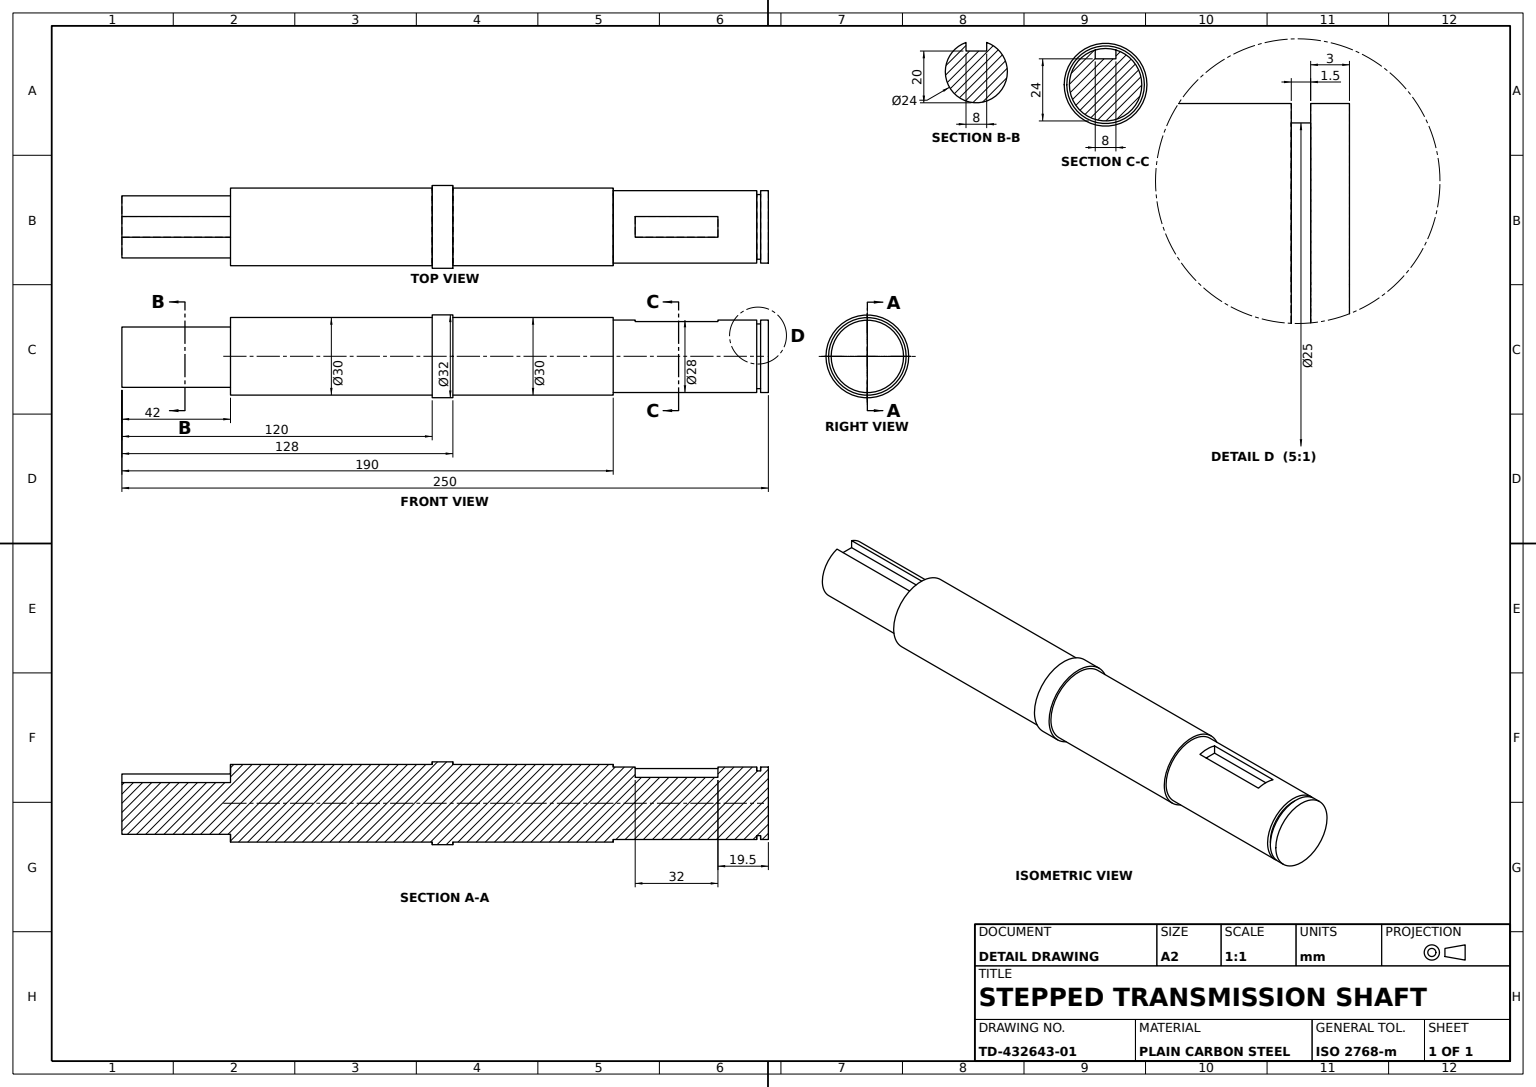
from build123d import *

# Parameters (mm, degrees)
KEYWAY_1_SKETCH_W  = 42
KEYWAY_1_SKETCH_H  = 8
KEYWAY_1_CUT_DEPTH = 4
KEYWAY_2_SKETCH_W  = 32
KEYWAY_2_SKETCH_H  = 8
KEYWAY_2_CUT_DEPTH = 4


with BuildPart() as part:
    # Shaft Profile Sketch → Stepped Shaft Body (revolve)
    with BuildSketch(Plane.XY, mode=Mode.PRIVATE) as stepped_shaft_body_sk:
        Polygon((0, 0), (0, 12), (42, 12), (42, 15), (120, 15), (120, 16), (128, 16), (128, 15), (190, 15), (190, 14), (245.5, 14), (245.5, 12.5), (247, 12.5), (247, 14), (250, 14), (250, 0), align=None)
    revolve(stepped_shaft_body_sk.sketch.rotate(Axis((0, 0, 0), (1, 0, 0)), 90), axis=Axis((0, 0, 0), (1, 0, 0)))

    # Keyway 1 Sketch → Keyway 1 Cut (cut)
    with BuildSketch(Plane(origin=(0, 12, 0), x_dir=(1, 0, 0), z_dir=(0, 1, 0))):
        with Locations((21, 0)):
            Rectangle(KEYWAY_1_SKETCH_W, KEYWAY_1_SKETCH_H)
    extrude(amount=-KEYWAY_1_CUT_DEPTH, mode=Mode.SUBTRACT)

    # Keyway 2 Sketch → Keyway 2 Cut (cut)
    with BuildSketch(Plane(origin=(0, 14, 0), x_dir=(1, 0, 0), z_dir=(0, 1, 0))):
        with Locations((214.5, 0)):
            Rectangle(KEYWAY_2_SKETCH_W, KEYWAY_2_SKETCH_H)
    extrude(amount=-KEYWAY_2_CUT_DEPTH, mode=Mode.SUBTRACT)


solid = part.part
